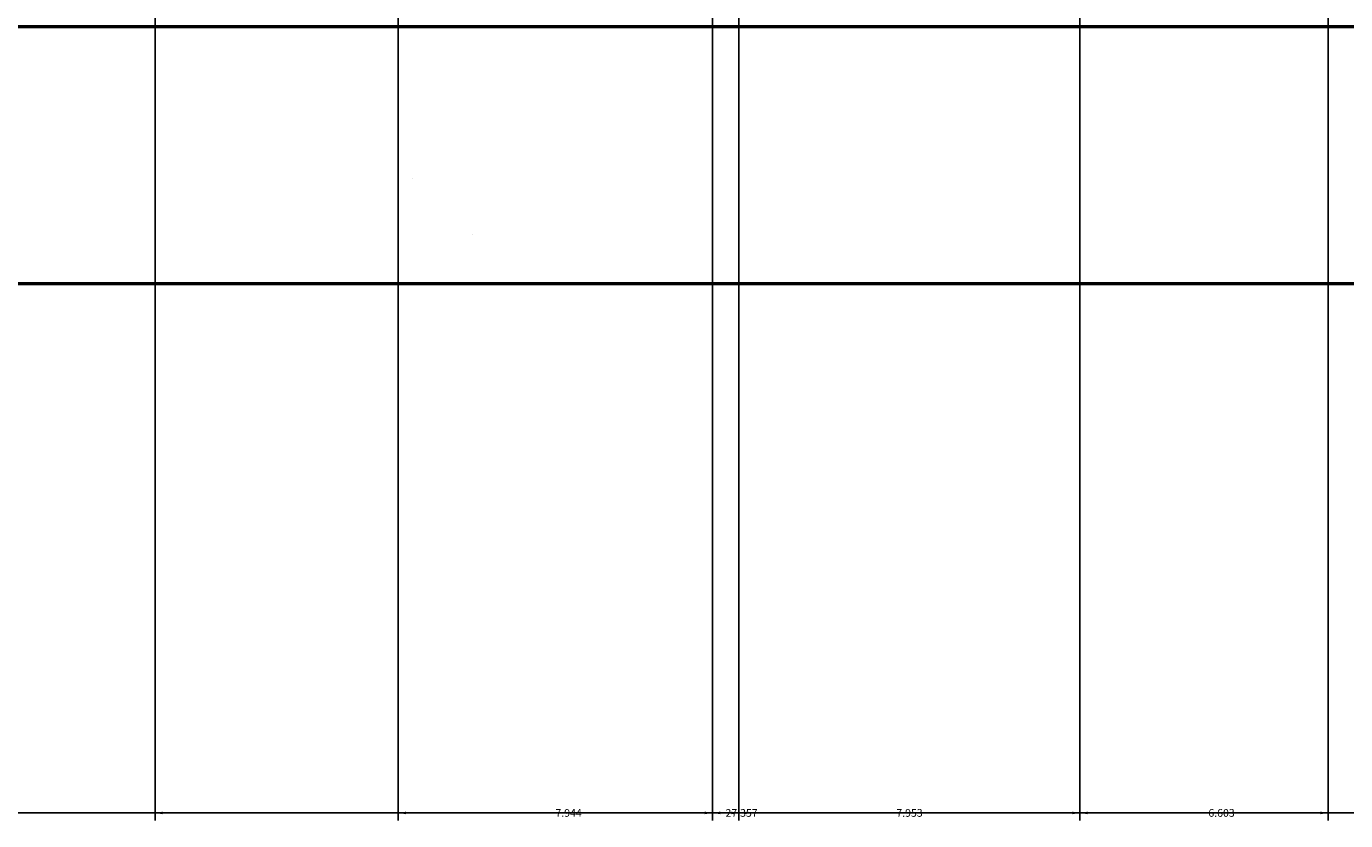
# Model space of a CAD drawing. Units: inches. Extents: x 2812 to 3051, y 1398 to 1659.
# Tile 13 of 65: x 2880 to 2911, y 1398 to 1416. Entities that reach past the tile are written whole.
import ezdxf

# ---------------------------------------------------------------- set-up
doc = ezdxf.new("R2010")
doc.units = ezdxf.units.IN
for name, color, linetype, lineweight in [('A-ANNO-DIMS', 2, 'Continuous', 18), ('S-CONC', 7, 'Continuous', 50), ('S-CONC-PATT', 8, 'Continuous', 18)]:
    doc.layers.add(name, color=color, linetype=linetype, lineweight=lineweight)
doc.styles.get("Standard").update_dxf_attribs({"font": 'arial.ttf'})
doc.dimstyles.get("Standard").update_dxf_attribs({"dimtxt": 0.18, "dimasz": 0.18, "dimexe": 0.18, "dimexo": 0.0625, "dimgap": 0.09, "dimtad": 0, "dimtih": 1, "dimtoh": 1, "dimdec": 4, "dimzin": 0, "dimdsep": 46, "dimtxsty": 'Standard', "dimcen": 0.09, "dimadec": 0, "dimazin": 0, "dimtfac": 1, "dimtdec": 4, "dimtofl": 0, "dimtmove": 0, "dimatfit": 3, "dimfxl": 1, "dimtolj": 1, "dimtzin": 0, "dimarcsym": 0})

# ---------------------------------------------------------------- blocks, each defined once
blk = doc.blocks.new('*D29')
at = {"layer": 'A-ANNO-DIMS', "color": 0, "lineweight": -2, "transparency": 16777216}
for p, q in [((2910.742, 1598.757), (2910.742, 1397.505)), ((2883.385, 1559.757), (2883.385, 1397.505)), ((2883.565, 1397.685), (2896.598, 1397.685)), ((2910.562, 1397.685), (2897.528, 1397.685))]:
    blk.add_line(p, q, dxfattribs=at)
at = {"layer": 'A-ANNO-DIMS', "color": 0, "transparency": 16777216}
for points in [[(2883.565, 1397.715), (2883.565, 1397.655), (2883.385, 1397.685)], [(2910.562, 1397.715), (2910.562, 1397.655), (2910.742, 1397.685)]]:
    blk.add_solid(points, dxfattribs=at)
at = {"layer": 'Defpoints', "color": 0, "transparency": 16777216}
for p in [(2910.742, 1598.82), (2883.385, 1559.82), (2910.742, 1397.685)]:
    blk.add_point(p, dxfattribs=at)
at = {"layer": 'A-ANNO-DIMS', "color": 0, "transparency": 16777216, "insert": (2897.063, 1397.685), "char_height": 0.18, "attachment_point": 5}
blk.add_mtext('\\A1;27.357', dxfattribs=at)
blk = doc.blocks.new('*D44')
at = {"layer": 'A-ANNO-DIMS', "color": 0, "lineweight": -2, "transparency": 16777216}
for p, q in [((2850.748, 1487.973), (2850.748, 1397.505)), ((2896.385, 1487.973), (2896.385, 1397.505)), ((2850.928, 1397.685), (2873.17, 1397.685)), ((2896.205, 1397.685), (2873.964, 1397.685))]:
    blk.add_line(p, q, dxfattribs=at)
at = {"layer": 'A-ANNO-DIMS', "color": 0, "transparency": 16777216}
for points in [[(2850.928, 1397.715), (2850.928, 1397.655), (2850.748, 1397.685)], [(2896.205, 1397.715), (2896.205, 1397.655), (2896.385, 1397.685)]]:
    blk.add_solid(points, dxfattribs=at)
at = {"layer": 'Defpoints', "color": 0, "transparency": 16777216}
for p in [(2850.748, 1488.035), (2896.385, 1488.035), (2896.385, 1397.685)]:
    blk.add_point(p, dxfattribs=at)
at = {"layer": 'A-ANNO-DIMS', "color": 0, "transparency": 16777216, "insert": (2873.567, 1397.685), "char_height": 0.18, "attachment_point": 5}
blk.add_mtext('\\A1;45.64', dxfattribs=at)
blk = doc.blocks.new('*D45')
at = {"layer": 'A-ANNO-DIMS', "color": 0, "lineweight": -2, "transparency": 16777216}
for p, q in [((2896.385, 1487.973), (2896.385, 1397.505)), ((2941.385, 1487.973), (2941.385, 1397.505)), ((2896.565, 1397.685), (2918.662, 1397.685)), ((2941.205, 1397.685), (2919.108, 1397.685))]:
    blk.add_line(p, q, dxfattribs=at)
at = {"layer": 'A-ANNO-DIMS', "color": 0, "transparency": 16777216}
for points in [[(2896.565, 1397.715), (2896.565, 1397.655), (2896.385, 1397.685)], [(2941.205, 1397.715), (2941.205, 1397.655), (2941.385, 1397.685)]]:
    blk.add_solid(points, dxfattribs=at)
at = {"layer": 'Defpoints', "color": 0, "transparency": 16777216}
for p in [(2896.385, 1488.035), (2941.385, 1488.035), (2941.385, 1397.685)]:
    blk.add_point(p, dxfattribs=at)
at = {"layer": 'A-ANNO-DIMS', "color": 0, "transparency": 16777216, "insert": (2918.885, 1397.685), "char_height": 0.18, "attachment_point": 5}
blk.add_mtext('\\A1;45', dxfattribs=at)
blk = doc.blocks.new('*D60')
at = {"layer": 'A-ANNO-DIMS', "color": 0, "lineweight": -2, "transparency": 16777216}
for p, q in [((2889.058, 1466.34), (2889.058, 1397.505)), ((2897.002, 1457.364), (2897.002, 1397.505)), ((2889.238, 1397.685), (2892.637, 1397.685)), ((2896.822, 1397.685), (2893.422, 1397.685))]:
    blk.add_line(p, q, dxfattribs=at)
at = {"layer": 'A-ANNO-DIMS', "color": 0, "transparency": 16777216}
for points in [[(2889.238, 1397.715), (2889.238, 1397.655), (2889.058, 1397.685)], [(2896.822, 1397.715), (2896.822, 1397.655), (2897.002, 1397.685)]]:
    blk.add_solid(points, dxfattribs=at)
at = {"layer": 'Defpoints', "color": 0, "transparency": 16777216}
for p in [(2889.058, 1466.402), (2897.002, 1457.426), (2897.002, 1397.685)]:
    blk.add_point(p, dxfattribs=at)
at = {"layer": 'A-ANNO-DIMS', "color": 0, "transparency": 16777216, "insert": (2893.03, 1397.685), "char_height": 0.18, "attachment_point": 5}
blk.add_mtext('\\A1;7.944', dxfattribs=at)
blk = doc.blocks.new('*D61')
at = {"layer": 'A-ANNO-DIMS', "color": 0, "lineweight": -2, "transparency": 16777216}
for p, q in [((2897.002, 1457.364), (2897.002, 1397.505)), ((2904.955, 1447.364), (2904.955, 1397.505)), ((2897.182, 1397.685), (2900.586, 1397.685)), ((2904.775, 1397.685), (2901.372, 1397.685))]:
    blk.add_line(p, q, dxfattribs=at)
at = {"layer": 'A-ANNO-DIMS', "color": 0, "transparency": 16777216}
for points in [[(2897.182, 1397.715), (2897.182, 1397.655), (2897.002, 1397.685)], [(2904.775, 1397.715), (2904.775, 1397.655), (2904.955, 1397.685)]]:
    blk.add_solid(points, dxfattribs=at)
at = {"layer": 'Defpoints', "color": 0, "transparency": 16777216}
for p in [(2897.002, 1457.426), (2904.955, 1447.426), (2904.955, 1397.685)]:
    blk.add_point(p, dxfattribs=at)
at = {"layer": 'A-ANNO-DIMS', "color": 0, "transparency": 16777216, "insert": (2900.979, 1397.685), "char_height": 0.18, "attachment_point": 5}
blk.add_mtext('\\A1;7.953', dxfattribs=at)
blk = doc.blocks.new('*D62')
at = {"layer": 'A-ANNO-DIMS', "color": 0, "lineweight": -2, "transparency": 16777216}
for p, q in [((2904.955, 1447.364), (2904.955, 1397.505)), ((2911.558, 1437.364), (2911.558, 1397.505)), ((2905.135, 1397.685), (2907.862, 1397.685)), ((2911.378, 1397.685), (2908.651, 1397.685))]:
    blk.add_line(p, q, dxfattribs=at)
at = {"layer": 'A-ANNO-DIMS', "color": 0, "transparency": 16777216}
for points in [[(2905.135, 1397.715), (2905.135, 1397.655), (2904.955, 1397.685)], [(2911.378, 1397.715), (2911.378, 1397.655), (2911.558, 1397.685)]]:
    blk.add_solid(points, dxfattribs=at)
at = {"layer": 'Defpoints', "color": 0, "transparency": 16777216}
for p in [(2904.955, 1447.426), (2911.558, 1437.426), (2911.558, 1397.685)]:
    blk.add_point(p, dxfattribs=at)
at = {"layer": 'A-ANNO-DIMS', "color": 0, "transparency": 16777216, "insert": (2908.256, 1397.685), "char_height": 0.18, "attachment_point": 5}
blk.add_mtext('\\A1;6.603', dxfattribs=at)

msp = doc.modelspace()

# ---------------------------------------------------------------- hatches: boundary and pattern name
at = {"layer": 'S-CONC-PATT'}
h = msp.add_hatch(dxfattribs=at)
h.set_pattern_fill('AR-SAND', color=256, scale=0.3)
h.paths.add_polyline_path([(3036.3849, 1416.0354), (3027.3849, 1416.0354), (2826.3849, 1416.0354), (2826.3849, 1410.0354), (2835.3849, 1410.0354), (3036.3849, 1410.0354)])
h.paths.add_polyline_path([(2970.3849, 1488.0354), (2969.3849, 1488.0354), (2941.3849, 1488.0354), (2941.3849, 1482.0354), (2970.3849, 1482.0354)])
h.paths.add_polyline_path([(3036.3849, 1488.0354), (3035.3849, 1488.0354), (3006.3849, 1488.0354), (3006.3849, 1482.0354), (3027.3849, 1482.0354), (3036.3849, 1482.0354)])
h.paths.add_polyline_path([(3034.3849, 1490.0354), (3008.3849, 1490.0354), (3008.3849, 1489.0354), (3034.3849, 1489.0354)])
h.paths.add_polyline_path([(3035.3849, 1489.0354), (3034.3849, 1489.0354), (3007.3849, 1489.0354), (3007.3849, 1488.0354), (3035.3849, 1488.0354)])
h.paths.add_polyline_path([(2968.3849, 1490.0354), (2943.3849, 1490.0354), (2943.3849, 1489.0354), (2968.3849, 1489.0354)])
h.paths.add_polyline_path([(2969.3849, 1489.0354), (2968.3849, 1489.0354), (2942.3849, 1489.0354), (2942.3849, 1488.0354), (2969.3849, 1488.0354)])
h.paths.add_polyline_path([(2896.3849, 1488.0354), (2826.3849, 1488.0354), (2826.3849, 1482.0354), (2896.3849, 1482.0354)])
h.paths.add_polyline_path([(2895.3849, 1489.0354), (2894.3849, 1489.0354), (2827.3849, 1489.0354), (2827.3849, 1488.0354), (2895.3849, 1488.0354)])
h.paths.add_polyline_path([(2894.3849, 1490.0354), (2828.3849, 1490.0354), (2828.3849, 1489.0354), (2894.3849, 1489.0354)])
h = msp.add_hatch(dxfattribs=at)
h.set_pattern_fill('AR-CONC', color=256, scale=0.3)
h.paths.add_polyline_path([(3036.3849, 1416.0354), (3027.3849, 1416.0354), (2826.3849, 1416.0354), (2826.3849, 1410.0354), (2835.3849, 1410.0354), (3036.3849, 1410.0354)])

# ---------------------------------------------------------------- linework, layer by layer
at = {"layer": 'S-CONC'}
for p, q in [((2826.3849, 1416.0354), (3027.3849, 1416.0354)), ((2835.3849, 1410.0354), (3036.3849, 1410.0354))]:
    msp.add_line(p, q, dxfattribs=at)

# ---------------------------------------------------------------- dimensions: what is measured, and where the dimension line sits
at = {"layer": 'A-ANNO-DIMS'}
for base, p1, p2, override, picture, middle in [((2910.7415, 1397.6854), (2883.3849, 1559.82), (2910.7415, 1598.82), {"dimdec": 3, "dimlfac": 1, "dimrnd": 0, "dimzin": 0, "dimdsep": 46, "dimlunit": 2}, '*D29', (2897.0632, 1397.6854)), ((2896.3849, 1397.6854), (2850.7485, 1488.0354), (2896.3849, 1488.0354), {"dimdec": 2, "dimlfac": 1, "dimrnd": 0, "dimzin": 0, "dimdsep": 46, "dimlunit": 2}, '*D44', (2873.5667, 1397.6854)), ((2941.3849, 1397.6854), (2896.3849, 1488.0354), (2941.3849, 1488.0354), {"dimdec": 0, "dimlfac": 1, "dimrnd": 0, "dimzin": 0, "dimdsep": 46, "dimlunit": 2}, '*D45', (2918.8849, 1397.6854)), ((2897.0021, 1397.6854), (2889.0577, 1466.4024), (2897.0021, 1457.4265), {"dimdec": 3, "dimlfac": 1, "dimrnd": 0, "dimzin": 0, "dimdsep": 46, "dimlunit": 2}, '*D60', (2893.0299, 1397.6854)), ((2904.9551, 1397.6854), (2897.0021, 1457.4265), (2904.9551, 1447.4265), {"dimdec": 3, "dimlfac": 1, "dimrnd": 0, "dimzin": 0, "dimdsep": 46, "dimlunit": 2}, '*D61', (2900.9786, 1397.6854)), ((2911.5577, 1397.6854), (2904.9551, 1447.4265), (2911.5577, 1437.4265), {"dimdec": 3, "dimlfac": 1, "dimrnd": 0, "dimzin": 0, "dimdsep": 46, "dimlunit": 2}, '*D62', (2908.2564, 1397.6854))]:
    dim = msp.add_linear_dim(base=base, p1=p1, p2=p2, dimstyle='Standard', override=override, dxfattribs=at)
    dim.commit()
    dim.dimension.update_dxf_attribs({"geometry": picture, "text_midpoint": middle})

doc.saveas('drawing.dxf')
